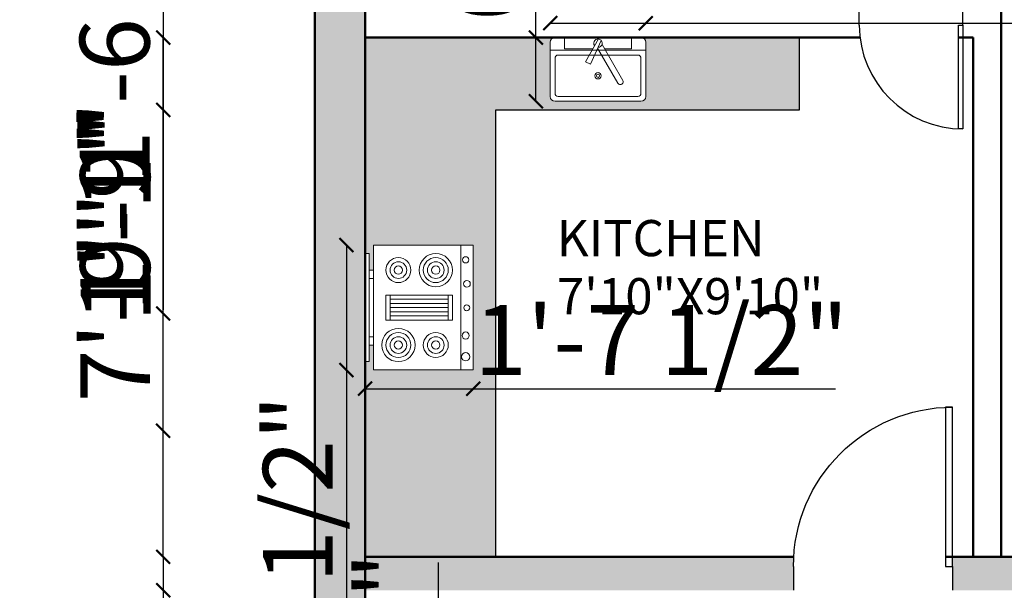
# Model space of a CAD drawing. Units: inches. Extents: x 2419 to 2878, y 1068 to 1713.
# Tile 14 of 20: x 2419 to 2595, y 1409 to 1511. Entities that reach past the tile are written whole.
import ezdxf

# ---------------------------------------------------------------- set-up
doc = ezdxf.new("R2010")
doc.units = ezdxf.units.IN
for name, color, linetype, lineweight in [('A-ANNO-DIMS', 2, 'Continuous', 18), ('A-AREA-IDEN', 7, 'Continuous', 18), ('A-DOOR', 4, 'Continuous', 25), ('A-EQPM', 9, 'Continuous', 18), ('A-FLOR-CASE', 8, 'Continuous', 25), ('A-FLOR-FIXT', 8, 'Continuous', 18), ('A-FLOR-PRKG-PATT', 1, 'Continuous', 13), ('A-FURN-PATT', 254, 'Continuous', 13), ('A-WALL', 7, 'Continuous', 50)]:
    doc.layers.add(name, color=color, linetype=linetype, lineweight=lineweight)
for name, color, linetype, lineweight, true_color in [('A-FLOR-CASE-PATT', 254, 'Continuous', 13, 0xcecce6), ('A-FLOR-FIXT-PATT', 254, 'Continuous', 13, 0xd7ebd2), ('A-WALL-PATT', 18, 'Continuous', 13, 0x000000)]:
    doc.layers.add(name, color=color, linetype=linetype, lineweight=lineweight, true_color=true_color)
doc.styles.get("Standard").update_dxf_attribs({"font": 'arial.ttf'})
doc.dimstyles.new('ISO-25', dxfattribs={"dimtxt": 12.5, "dimasz": 2.5, "dimexe": 1.25, "dimexo": 0.625, "dimtad": 1, "dimdec": 0, "dimlunit": 4, "dimtxsty": 'Standard', "dimblk": 'ARCHTICK', "dimcen": 2.5, "dimse1": 1, "dimse2": 1, "dimclrd": 4, "dimadec": 0, "dimazin": 0, "dimtfac": 1, "dimtdec": 0, "dimtmove": 0, "dimatfit": 3, "dimfxl": 1, "dimarcsym": 0})

# ---------------------------------------------------------------- blocks, each defined once
blk = doc.blocks.new('Range-Oven - 30 in top')
for p, q in [((0, -3), (30, -3)), ((12, -6), (18, -6)), ((13, -20), (13, -6)), ((14, -6), (14, -20)), ((15, -20), (15, -6)), ((16, -6), (16, -20)), ((17, -20), (17, -6)), ((18, -20), (12, -20)), ((6, -24), (6, -25)), ((8, -25), (8, -24)), ((22, -25), (22, -24)), ((24, -24), (24, -25))]:
    blk.add_line(p, q)
for points in [[(0, -24), (0, 0), (30, 0), (30, -24)], [(12, -21), (12, -5), (18, -5), (18, -21)], [(2, -26), (2, -25), (28, -25), (28, -26)]]:
    blk.add_lwpolyline(points, close=True)
for centre, radius in [((6, -9), 4), ((6, -9), 3), ((6, -9), 2), ((24, -9), 3), ((24, -9), 2), ((6, -9), 1), ((24, -9), 1), ((24, -18), 4), ((6, -18), 3), ((6, -18), 2), ((24, -18), 3), ((24, -18), 2), ((6, -18), 1), ((24, -18), 1)]:
    blk.add_circle(centre, radius)
blk = doc.blocks.new('Faucet - single handle top')
for p, q in [((0.08, -0.26), (-2.26, -4.34)), ((-1.37, -4.79), (0.55, -0.5)), ((4.43, -7.68), (0.72, -1.24)), ((-0.06, -1.9), (3.57, -8.18)), ((-2.26, -4.34), (-1.37, -4.79))]:
    blk.add_line(p, q)
for points in [[(-0.92, -2), (-6, -2), (-6, 0), (6, 0), (6, -2), (1.16, -2)], [(-0.01, -2), (-0.12, -2)]]:
    blk.add_lwpolyline(points)
for centre, radius, start, end in [((0, -1), 0.75, 269.2246, 216.2304), ((4, -7.93), 0.5, 210, 30)]:
    blk.add_arc(centre, radius, start, end)
blk = doc.blocks.new('Sink-single - 30 in top')
blk.add_line((-15, -3.999996), (15, -3.999996))
for points in [[(-13.5, 0), (13.5, 0)], [(-15, -18.499996), (-15, -1.5)], [(15, -1.5), (15, -18.499996)], [(-12.5, -5.499996), (12.5, -5.499996)], [(-13.5, -17.499996), (-13.5, -6.499996)], [(13.5, -6.499996), (13.5, -17.499996)], [(12.5, -18.499996), (-12.5, -18.499996)], [(13.5, -19.999996), (-13.5, -19.999996)]]:
    blk.add_lwpolyline(points)
for radius in [1, 0.5]:
    blk.add_circle((0, -11.999996), radius)
for centre, radius, start, end in [((-13.5, -1.5), 1.5, 90, 180), ((13.5, -1.5), 1.5, 0, 90), ((-12.5, -6.499996), 1, 90, 180), ((12.5, -6.499996), 1, 0, 90), ((-13.5, -18.499996), 1.5, 180, 270), ((-12.5, -17.499996), 1, 180, 270), ((12.5, -17.499996), 1, 270, 0), ((13.5, -18.499996), 1.5, 270, 0)]:
    blk.add_arc(centre, radius, start, end)
blk = doc.blocks.new('*U3')
for p, q in [((0, 0), (0, -6)), ((40, 0), (40, -6))]:
    blk.add_line(p, q)
blk.add_lwpolyline([(0, 0), (0, 40), (1.75, 40), (1.75, 0)], close=True)
blk.add_arc((0, 0), 40, 0, 90)
blk = doc.blocks.new('_ArchTick')
at = {"color": 0, "linetype": 'ByBlock', "const_width": 0.15}
blk.add_lwpolyline([(-0.5, -0.5), (0.5, 0.5)], dxfattribs=at)
blk = doc.blocks.new('*D22')
at = {"layer": 'A-ANNO-DIMS', "color": 4, "lineweight": -2, "transparency": 16777216}
for p, q in [((2513.7, 1510.38), (2530.82, 1510.38)), ((2530.82, 1510.38), (2656.31, 1510.38))]:
    blk.add_line(p, q, dxfattribs=at)
at = {"layer": 'Defpoints', "color": 0, "transparency": 16777216}
for p in [(2530.82, 1510.38), (2513.7, 1507.81), (2530.82, 1507.81)]:
    blk.add_point(p, dxfattribs=at)
at = {"layer": 'A-ANNO-DIMS', "color": 4, "lineweight": -2, "transparency": 16777216, "xscale": 2.5, "yscale": 2.5, "zscale": 2.5, "rotation": 180}
blk.add_blockref('_ArchTick', (2513.7, 1510.38), dxfattribs=at)
at = {"layer": 'A-ANNO-DIMS', "color": 4, "lineweight": -2, "transparency": 16777216, "xscale": 2.5, "yscale": 2.5, "zscale": 2.5}
blk.add_blockref('_ArchTick', (2530.82, 1510.38), dxfattribs=at)
at = {"layer": 'A-ANNO-DIMS', "color": 0, "transparency": 16777216, "insert": (2594.82, 1517.47), "char_height": 12.5, "attachment_point": 5}
blk.add_mtext('SINK 1\'-5" TYP.', dxfattribs=at)
blk = doc.blocks.new('*D23')
at = {"layer": 'A-ANNO-DIMS', "color": 4, "lineweight": -2, "transparency": 16777216}
for p, q in [((2511.14, 1507.81), (2511.14, 1626.6)), ((2511.14, 1496.4), (2511.14, 1507.81))]:
    blk.add_line(p, q, dxfattribs=at)
at = {"layer": 'Defpoints', "color": 0, "transparency": 16777216}
for p in [(2511.14, 1507.81), (2513.7, 1507.81), (2513.7, 1496.4)]:
    blk.add_point(p, dxfattribs=at)
at = {"layer": 'A-ANNO-DIMS', "color": 4, "lineweight": -2, "transparency": 16777216, "xscale": 2.5, "yscale": 2.5, "zscale": 2.5}
for p, rotation in [((2511.14, 1507.81), 90), ((2511.14, 1496.4), 270)]:
    blk.add_blockref('_ArchTick', p, dxfattribs=dict(at, rotation=rotation))
at = {"layer": 'A-ANNO-DIMS', "color": 0, "transparency": 16777216, "insert": (2504.05, 1568.45), "char_height": 12.5, "attachment_point": 5, "rotation": 90}
blk.add_mtext('0\'-11 1/2" TYP.', dxfattribs=at)
blk = doc.blocks.new('*D27')
at = {"layer": 'A-ANNO-DIMS', "color": 4, "lineweight": -2, "transparency": 16777216}
for p, q in [((2493.67, 1347.69), (2493.67, 1413.78)), ((2493.67, 1311.01), (2493.67, 1347.69))]:
    blk.add_line(p, q, dxfattribs=at)
at = {"layer": 'Defpoints', "color": 0, "transparency": 16777216}
for p in [(2493.67, 1347.69), (2502.77, 1347.69), (2502.77, 1311.01)]:
    blk.add_point(p, dxfattribs=at)
at = {"layer": 'A-ANNO-DIMS', "color": 4, "lineweight": -2, "transparency": 16777216, "xscale": 2.5, "yscale": 2.5, "zscale": 2.5}
for p, rotation in [((2493.67, 1347.69), 90), ((2493.67, 1311.01), 270)]:
    blk.add_blockref('_ArchTick', p, dxfattribs=dict(at, rotation=rotation))
at = {"layer": 'A-ANNO-DIMS', "color": 0, "transparency": 16777216, "insert": (2486.57, 1381.99), "char_height": 12.5, "attachment_point": 5, "rotation": 90}
blk.add_mtext('3\'-0 1/2"', dxfattribs=at)
blk = doc.blocks.new('*D28')
at = {"layer": 'A-ANNO-DIMS', "color": 4, "lineweight": -2, "transparency": 16777216}
for p, q in [((2477.16, 1470.63), (2477.16, 1448.27)), ((2477.16, 1448.27), (2477.16, 1306.15))]:
    blk.add_line(p, q, dxfattribs=at)
at = {"layer": 'Defpoints', "color": 0, "transparency": 16777216}
for p in [(2480.51, 1470.63), (2477.16, 1448.27), (2480.51, 1448.27)]:
    blk.add_point(p, dxfattribs=at)
at = {"layer": 'A-ANNO-DIMS', "color": 4, "lineweight": -2, "transparency": 16777216, "xscale": 2.5, "yscale": 2.5, "zscale": 2.5}
for p, rotation in [((2477.16, 1470.63), 90), ((2477.16, 1448.27), 270)]:
    blk.add_blockref('_ArchTick', p, dxfattribs=dict(at, rotation=rotation))
at = {"layer": 'A-ANNO-DIMS', "color": 0, "transparency": 16777216, "insert": (2470.07, 1375.96), "char_height": 12.5, "attachment_point": 5, "rotation": 90}
blk.add_mtext('RANGE 1\'-10 1/2"', dxfattribs=at)
blk = doc.blocks.new('*D29')
at = {"layer": 'A-ANNO-DIMS', "color": 4, "lineweight": -2, "transparency": 16777216}
for p, q in [((2480.51, 1444.92), (2499.89, 1444.92)), ((2499.89, 1444.92), (2564.82, 1444.92))]:
    blk.add_line(p, q, dxfattribs=at)
at = {"layer": 'Defpoints', "color": 0, "transparency": 16777216}
for p in [(2480.51, 1448.27), (2499.89, 1448.27), (2499.89, 1444.92)]:
    blk.add_point(p, dxfattribs=at)
at = {"layer": 'A-ANNO-DIMS', "color": 4, "lineweight": -2, "transparency": 16777216, "xscale": 2.5, "yscale": 2.5, "zscale": 2.5, "rotation": 180}
blk.add_blockref('_ArchTick', (2480.51, 1444.92), dxfattribs=at)
at = {"layer": 'A-ANNO-DIMS', "color": 4, "lineweight": -2, "transparency": 16777216, "xscale": 2.5, "yscale": 2.5, "zscale": 2.5}
blk.add_blockref('_ArchTick', (2499.89, 1444.92), dxfattribs=at)
at = {"layer": 'A-ANNO-DIMS', "color": 0, "transparency": 16777216, "insert": (2533.61, 1452.01), "char_height": 12.5, "attachment_point": 5}
blk.add_mtext('1\'-7 1/2"', dxfattribs=at)
blk = doc.blocks.new('*D48')
at = {"layer": 'A-ANNO-DIMS', "color": 4, "lineweight": -2, "transparency": 16777216}
for p, q in [((2444.31, 1567.55), (2444.31, 1548.96)), ((2444.31, 1548.96), (2444.31, 1484.03))]:
    blk.add_line(p, q, dxfattribs=at)
at = {"layer": 'Defpoints', "color": 0, "transparency": 16777216}
for p in [(2725.51, 1567.55), (2444.31, 1548.96), (2725.51, 1548.96)]:
    blk.add_point(p, dxfattribs=at)
at = {"layer": 'A-ANNO-DIMS', "color": 4, "lineweight": -2, "transparency": 16777216, "xscale": 2.5, "yscale": 2.5, "zscale": 2.5}
for p, rotation in [((2444.31, 1567.55), 90), ((2444.31, 1548.96), 270)]:
    blk.add_blockref('_ArchTick', p, dxfattribs=dict(at, rotation=rotation))
at = {"layer": 'A-ANNO-DIMS', "color": 0, "transparency": 16777216, "insert": (2437.23, 1515.25), "char_height": 12.5, "attachment_point": 5, "rotation": 90}
blk.add_mtext('1\'-6 1/2"', dxfattribs=at)
blk = doc.blocks.new('*D50')
at = {"layer": 'A-ANNO-DIMS', "color": 4, "lineweight": -2, "transparency": 16777216}
for p, q in [((2444.31, 1458.39), (2444.31, 1494.19)), ((2444.31, 1437.39), (2444.31, 1458.39))]:
    blk.add_line(p, q, dxfattribs=at)
at = {"layer": 'Defpoints', "color": 0, "transparency": 16777216}
for p in [(2444.31, 1458.39), (2763.51, 1458.39), (2763.51, 1437.39)]:
    blk.add_point(p, dxfattribs=at)
at = {"layer": 'A-ANNO-DIMS', "color": 4, "lineweight": -2, "transparency": 16777216, "xscale": 2.5, "yscale": 2.5, "zscale": 2.5}
for p, rotation in [((2444.31, 1458.39), 90), ((2444.31, 1437.39), 270)]:
    blk.add_blockref('_ArchTick', p, dxfattribs=dict(at, rotation=rotation))
at = {"layer": 'A-ANNO-DIMS', "color": 0, "transparency": 16777216, "insert": (2437.31, 1477.54), "char_height": 12.5, "attachment_point": 5, "rotation": 90}
blk.add_mtext('1\'-9"', dxfattribs=at)
blk = doc.blocks.new('*D55')
at = {"layer": 'A-ANNO-DIMS', "color": 4, "lineweight": -2, "transparency": 16777216}
for p, q in [((2444.31, 1414.81), (2444.31, 1408.81)), ((2444.31, 1408.81), (2444.31, 1371.83))]:
    blk.add_line(p, q, dxfattribs=at)
at = {"layer": 'Defpoints', "color": 0, "transparency": 16777216}
for p in [(2480.51, 1414.81), (2444.31, 1408.81), (2480.51, 1408.81)]:
    blk.add_point(p, dxfattribs=at)
at = {"layer": 'A-ANNO-DIMS', "color": 4, "lineweight": -2, "transparency": 16777216, "xscale": 2.5, "yscale": 2.5, "zscale": 2.5}
for p, rotation in [((2444.31, 1414.81), 90), ((2444.31, 1408.81), 270)]:
    blk.add_blockref('_ArchTick', p, dxfattribs=dict(at, rotation=rotation))
at = {"layer": 'A-ANNO-DIMS', "color": 0, "transparency": 16777216, "insert": (2437.31, 1389.07), "char_height": 12.5, "attachment_point": 5, "rotation": 90}
blk.add_mtext('0\'-6"', dxfattribs=at)
blk = doc.blocks.new('*D56')
at = {"layer": 'A-ANNO-DIMS', "color": 4, "lineweight": -2, "transparency": 16777216}
for p, q in [((2480.51, 1079.92), (2503.97, 1079.92)), ((2503.97, 1079.92), (2578.61, 1079.92))]:
    blk.add_line(p, q, dxfattribs=at)
at = {"layer": 'Defpoints', "color": 0, "transparency": 16777216}
for p in [(2480.51, 1507.81), (2503.97, 1494.85), (2503.97, 1079.92)]:
    blk.add_point(p, dxfattribs=at)
at = {"layer": 'A-ANNO-DIMS', "color": 4, "lineweight": -2, "transparency": 16777216, "xscale": 2.5, "yscale": 2.5, "zscale": 2.5, "rotation": 180}
blk.add_blockref('_ArchTick', (2480.51, 1079.92), dxfattribs=at)
at = {"layer": 'A-ANNO-DIMS', "color": 4, "lineweight": -2, "transparency": 16777216, "xscale": 2.5, "yscale": 2.5, "zscale": 2.5}
blk.add_blockref('_ArchTick', (2503.97, 1079.92), dxfattribs=at)
at = {"layer": 'A-ANNO-DIMS', "color": 0, "transparency": 16777216, "insert": (2542.54, 1087.01), "char_height": 12.5, "attachment_point": 5}
blk.add_mtext('1\'-11 1/2"', dxfattribs=at)
blk = doc.blocks.new('*D57')
at = {"layer": 'A-ANNO-DIMS', "color": 4, "lineweight": -2, "transparency": 16777216}
blk.add_line((2480.51, 1605.01), (2558.38, 1605.01), dxfattribs=at)
at = {"layer": 'Defpoints', "color": 0, "transparency": 16777216}
for p in [(2558.38, 1605.01), (2480.51, 1507.81), (2558.38, 1507.81)]:
    blk.add_point(p, dxfattribs=at)
at = {"layer": 'A-ANNO-DIMS', "color": 4, "lineweight": -2, "transparency": 16777216, "xscale": 2.5, "yscale": 2.5, "zscale": 2.5, "rotation": 180}
blk.add_blockref('_ArchTick', (2480.51, 1605.01), dxfattribs=at)
at = {"layer": 'A-ANNO-DIMS', "color": 4, "lineweight": -2, "transparency": 16777216, "xscale": 2.5, "yscale": 2.5, "zscale": 2.5}
blk.add_blockref('_ArchTick', (2558.38, 1605.01), dxfattribs=at)
at = {"layer": 'A-ANNO-DIMS', "color": 0, "transparency": 16777216, "insert": (2519.45, 1612.02), "char_height": 12.5, "attachment_point": 5}
blk.add_mtext('6\'-6"', dxfattribs=at)
blk = doc.blocks.new('*D58')
at = {"layer": 'A-ANNO-DIMS', "color": 4, "lineweight": -2, "transparency": 16777216}
for p, q in [((2444.31, 1507.81), (2444.31, 1494.85)), ((2444.31, 1494.85), (2444.31, 1459.05))]:
    blk.add_line(p, q, dxfattribs=at)
at = {"layer": 'Defpoints', "color": 0, "transparency": 16777216}
for p in [(2480.51, 1507.81), (2444.31, 1494.85), (2503.97, 1494.85)]:
    blk.add_point(p, dxfattribs=at)
at = {"layer": 'A-ANNO-DIMS', "color": 4, "lineweight": -2, "transparency": 16777216, "xscale": 2.5, "yscale": 2.5, "zscale": 2.5}
for p, rotation in [((2444.31, 1507.81), 90), ((2444.31, 1494.85), 270)]:
    blk.add_blockref('_ArchTick', p, dxfattribs=dict(at, rotation=rotation))
at = {"layer": 'A-ANNO-DIMS', "color": 0, "transparency": 16777216, "insert": (2437.41, 1475.7), "char_height": 12.5, "attachment_point": 5, "rotation": 90}
blk.add_mtext('1\'-1"', dxfattribs=at)
blk = doc.blocks.new('*D59')
at = {"layer": 'A-ANNO-DIMS', "color": 4, "lineweight": -2, "transparency": 16777216}
blk.add_line((2480.51, 1079.92), (2589.51, 1079.92), dxfattribs=at)
at = {"layer": 'Defpoints', "color": 0, "transparency": 16777216}
for p in [(2480.51, 1414.81), (2589.51, 1414.81), (2589.51, 1079.92)]:
    blk.add_point(p, dxfattribs=at)
at = {"layer": 'A-ANNO-DIMS', "color": 4, "lineweight": -2, "transparency": 16777216, "xscale": 2.5, "yscale": 2.5, "zscale": 2.5, "rotation": 180}
blk.add_blockref('_ArchTick', (2480.51, 1079.92), dxfattribs=at)
at = {"layer": 'A-ANNO-DIMS', "color": 4, "lineweight": -2, "transparency": 16777216, "xscale": 2.5, "yscale": 2.5, "zscale": 2.5}
blk.add_blockref('_ArchTick', (2589.51, 1079.92), dxfattribs=at)
at = {"layer": 'A-ANNO-DIMS', "color": 0, "transparency": 16777216, "insert": (2535.01, 1086.93), "char_height": 12.5, "attachment_point": 5}
blk.add_mtext('9\'-1"', dxfattribs=at)
blk = doc.blocks.new('*D60')
at = {"layer": 'A-ANNO-DIMS', "color": 4, "lineweight": -2, "transparency": 16777216}
blk.add_line((2444.31, 1414.81), (2444.31, 1507.81), dxfattribs=at)
at = {"layer": 'Defpoints', "color": 0, "transparency": 16777216}
for p in [(2444.31, 1507.81), (2480.51, 1507.81), (2480.51, 1414.81)]:
    blk.add_point(p, dxfattribs=at)
at = {"layer": 'A-ANNO-DIMS', "color": 4, "lineweight": -2, "transparency": 16777216, "xscale": 2.5, "yscale": 2.5, "zscale": 2.5}
for p, rotation in [((2444.31, 1507.81), 90), ((2444.31, 1414.81), 270)]:
    blk.add_blockref('_ArchTick', p, dxfattribs=dict(at, rotation=rotation))
at = {"layer": 'A-ANNO-DIMS', "color": 0, "transparency": 16777216, "insert": (2437.31, 1461.31), "char_height": 12.5, "attachment_point": 5, "rotation": 90}
blk.add_mtext('7\'-9"', dxfattribs=at)

msp = doc.modelspace()

# ---------------------------------------------------------------- hatches: boundary and pattern name
at = {"layer": 'A-FLOR-CASE-PATT'}
h = msp.add_hatch(color=256, dxfattribs=at)
h.dxf.hatch_style = 1
h.paths.add_polyline_path([(2503.97, 1494.85), (2558.38, 1494.85), (2558.38, 1507.81), (2529.96, 1507.81, -0.414214), (2530.82, 1506.96), (2530.82, 1497.26, -0.414214), (2529.96, 1496.4), (2514.56, 1496.4, -0.414214), (2513.7, 1497.26), (2513.7, 1506.96, -0.414214), (2514.56, 1507.81), (2480.51, 1507.81), (2480.51, 1469.14), (2481.26, 1469.14), (2481.26, 1466.16), (2482.01, 1466.16), (2482.01, 1470.63), (2499.89, 1470.63), (2499.89, 1448.27), (2482.01, 1448.27), (2482.01, 1452.74), (2481.26, 1452.74), (2481.26, 1449.76), (2480.51, 1449.76), (2480.51, 1414.81), (2503.97, 1414.81)])
at = {"layer": 'A-FLOR-FIXT-PATT'}
h = msp.add_hatch(color=256, dxfattribs=at)
h.dxf.hatch_style = 1
h.paths.add_polyline_path([(2771.51, 1458.39), (2763.51, 1458.39), (2763.51, 1437.39), (2771.51, 1437.39)])
h.paths.add_polyline_path([(2770.51, 1456.39, 0.5), (2769.51, 1457.39), (2765.51, 1457.39, 0.5), (2764.51, 1456.39), (2764.51, 1439.39, 0.5), (2765.51, 1438.39), (2769.51, 1438.39, 0.5), (2770.51, 1439.39)], flags=16)
h.paths.add_polyline_path([(2706.38, 1408.81), (2685.38, 1408.81), (2685.38, 1400.81), (2706.38, 1400.81)])
h.paths.add_polyline_path([(2704.38, 1401.81, 0.5), (2705.38, 1402.81), (2705.38, 1406.81, 0.5), (2704.38, 1407.81), (2687.38, 1407.81, 0.5), (2686.38, 1406.81), (2686.38, 1402.81, 0.5), (2687.38, 1401.81)], flags=16)
h.paths.add_polyline_path([(2574.48, 1207.45), (2633.94, 1207.45), (2633.94, 1217.37), (2574.48, 1217.37)], flags=9)
h.paths.add_polyline_path([(2574.45, 1217.83), (2610.47, 1217.83), (2610.47, 1227.88), (2574.45, 1227.88)], flags=9)
h.paths.add_polyline_path([(2672.43, 1304.02), (2718.62, 1304.02), (2718.62, 1313.94), (2672.43, 1313.94)], flags=9)
h.paths.add_polyline_path([(2672.4, 1314.4), (2750.13, 1314.4), (2750.13, 1324.45), (2672.4, 1324.45)], flags=9)
h.paths.add_polyline_path([(2500.43, 1374.44), (2544.8, 1374.44), (2544.8, 1384.36), (2500.43, 1384.36)], flags=9)
h.paths.add_polyline_path([(2500.41, 1384.82), (2566.08, 1384.82), (2566.08, 1394.87), (2500.41, 1394.87)], flags=9)
h.paths.add_polyline_path([(2738.93, 1376.75), (2778.27, 1376.75), (2778.27, 1386.67), (2738.93, 1386.67)], flags=9)
h.paths.add_polyline_path([(2659.12, 1357.8), (2703.49, 1357.8), (2703.49, 1367.72), (2659.12, 1367.72)], flags=9)
h.paths.add_polyline_path([(2659.1, 1368.18), (2694.11, 1368.18), (2694.11, 1378.23), (2659.1, 1378.23)], flags=9)
h.paths.add_polyline_path([(2730.12, 1466.07), (2769.46, 1466.07), (2769.46, 1475.99), (2730.12, 1475.99)], flags=9)
h.paths.add_polyline_path([(2730.1, 1476.45), (2765.12, 1476.45), (2765.12, 1486.5), (2730.1, 1486.5)], flags=9)
h.paths.add_polyline_path([(2730.38, 1518.65), (2761.48, 1518.65), (2761.48, 1528.57), (2730.38, 1528.57)], flags=9)
h.paths.add_polyline_path([(2730.36, 1529.03), (2780.96, 1529.03), (2780.96, 1539.07), (2730.36, 1539.07)], flags=9)
h.paths.add_polyline_path([(2629.32, 1455.19), (2688.78, 1455.19), (2688.78, 1465.11), (2629.32, 1465.11)], flags=9)
h.paths.add_polyline_path([(2629.3, 1465.57), (2681.9, 1465.57), (2681.9, 1475.62), (2629.3, 1475.62)], flags=9)
h.paths.add_polyline_path([(2513.23, 1456.48), (2562.63, 1456.48), (2562.63, 1466.4), (2513.23, 1466.4)], flags=9)
h.paths.add_polyline_path([(2513.21, 1466.86), (2556.26, 1466.86), (2556.26, 1476.91), (2513.21, 1476.91)], flags=9)
h.paths.add_polyline_path([(2488.87, 1521.54), (2519.97, 1521.54), (2519.97, 1531.46), (2488.87, 1531.46)], flags=9)
h.paths.add_polyline_path([(2536.55, 1543.51), (2580.92, 1543.51), (2580.92, 1553.43), (2536.55, 1553.43)], flags=9)
h.paths.add_polyline_path([(2536.56, 1553.92), (2573.53, 1553.92), (2573.53, 1563.8), (2536.56, 1563.8)], flags=9)
at = {"layer": 'A-FLOR-PRKG-PATT'}
h = msp.add_hatch(color=256, dxfattribs=at)
h.dxf.hatch_style = 1
edge = h.paths.add_edge_path()
edge.add_ellipse((2561.37, 1279.45), major_axis=(3.99, 0), ratio=0.842304, start_angle=0.6466, end_angle=90)
edge.add_line((2561.37, 1282.81), (2511.57, 1282.81))
edge.add_ellipse((2511.57, 1279.45), major_axis=(3.99, 0), ratio=0.842304, start_angle=90, end_angle=179.3534)
edge.add_ellipse((10560.89, 1188.62), major_axis=(-8054.03, 0), ratio=0.8423039, start_angle=-0.646554, end_angle=-0.628237)
edge.add_ellipse((2509.23, 1276.91), major_axis=(1.69, 0), ratio=0.842304, start_angle=179.3718, end_angle=248.4648)
edge.add_ellipse((10560.33, 1188.62), major_axis=(8052.29, 0), ratio=0.8423039, start_angle=179.353446, end_angle=179.381357, ccw=False)
edge.add_ellipse((2511.01, 1279.45), major_axis=(2.25, 0), ratio=0.842304, start_angle=90, end_angle=179.3534, ccw=False)
edge.add_line((2511.01, 1281.35), (2561.94, 1281.35))
edge.add_ellipse((2561.94, 1279.45), major_axis=(-2.25, 0), ratio=0.842304, start_angle=180.6466, end_angle=270, ccw=False)
edge.add_ellipse((-5487.38, 1188.62), major_axis=(8052.29, 0), ratio=0.8423039, start_angle=0.528271, end_angle=0.646554, ccw=False)
edge.add_ellipse((2563.71, 1276.91), major_axis=(-1.69, 0), ratio=0.842304, start_angle=111.5352, end_angle=180.6282)
edge.add_ellipse((-5487.95, 1188.62), major_axis=(-8054.03, 0), ratio=0.8423039, start_angle=180.628237, end_angle=180.646554)
edge = h.paths.add_edge_path()
edge.add_ellipse((2564.91, 1261.91), major_axis=(-1.12, 0), ratio=0.842304, start_angle=180, end_angle=270)
edge.add_line((2564.91, 1262.86), (2564.43, 1262.86))
edge.add_ellipse((-5487.38, 1188.62), major_axis=(8052.29, 0), ratio=0.8423039, start_angle=0.383867, end_angle=0.528271, ccw=False)
edge.add_line((2564.65, 1242.56), (2564.91, 1242.56))
edge.add_ellipse((2564.91, 1243.51), major_axis=(-1.12, 0), ratio=0.842304, start_angle=90, end_angle=180)
edge.add_line((2566.03, 1243.51), (2566.03, 1261.91))
edge = h.paths.add_edge_path()
edge.add_ellipse((2564.91, 1174.99), major_axis=(1.12, 0), ratio=0.842304, start_angle=0, end_angle=90)
edge.add_line((2564.91, 1175.94), (2564.89, 1175.94))
edge.add_ellipse((-5487.38, 1188.62), major_axis=(8052.29, 0), ratio=0.8423039, start_angle=-0.134987, end_angle=-0.090229, ccw=False)
edge.add_ellipse((2163.34, 1170.91), major_axis=(401.54, 0), ratio=0.842304, start_angle=-2.18, end_angle=-0.1356, ccw=False)
edge.add_line((2564.47, 1155.64), (2564.91, 1155.64))
edge.add_ellipse((2564.91, 1156.59), major_axis=(-1.12, 0), ratio=0.842304, start_angle=90, end_angle=180)
edge.add_line((2566.03, 1156.59), (2566.03, 1174.99))
h.paths.add_polyline_path([(2574.48, 1207.45), (2633.94, 1207.45), (2633.94, 1217.37), (2574.48, 1217.37)], flags=9)
h.paths.add_polyline_path([(2574.45, 1217.83), (2610.47, 1217.83), (2610.47, 1227.88), (2574.45, 1227.88)], flags=9)
h.paths.add_polyline_path([(2672.43, 1304.02), (2718.62, 1304.02), (2718.62, 1313.94), (2672.43, 1313.94)], flags=9)
h.paths.add_polyline_path([(2672.4, 1314.4), (2750.13, 1314.4), (2750.13, 1324.45), (2672.4, 1324.45)], flags=9)
h.paths.add_polyline_path([(2500.43, 1374.44), (2544.8, 1374.44), (2544.8, 1384.36), (2500.43, 1384.36)], flags=9)
h.paths.add_polyline_path([(2500.41, 1384.82), (2566.08, 1384.82), (2566.08, 1394.87), (2500.41, 1394.87)], flags=9)
h.paths.add_polyline_path([(2738.93, 1376.75), (2778.27, 1376.75), (2778.27, 1386.67), (2738.93, 1386.67)], flags=9)
h.paths.add_polyline_path([(2659.12, 1357.8), (2703.49, 1357.8), (2703.49, 1367.72), (2659.12, 1367.72)], flags=9)
h.paths.add_polyline_path([(2659.1, 1368.18), (2694.11, 1368.18), (2694.11, 1378.23), (2659.1, 1378.23)], flags=9)
h.paths.add_polyline_path([(2730.12, 1466.07), (2769.46, 1466.07), (2769.46, 1475.99), (2730.12, 1475.99)], flags=9)
h.paths.add_polyline_path([(2730.1, 1476.45), (2765.12, 1476.45), (2765.12, 1486.5), (2730.1, 1486.5)], flags=9)
h.paths.add_polyline_path([(2730.38, 1518.65), (2761.48, 1518.65), (2761.48, 1528.57), (2730.38, 1528.57)], flags=9)
h.paths.add_polyline_path([(2730.36, 1529.03), (2780.96, 1529.03), (2780.96, 1539.07), (2730.36, 1539.07)], flags=9)
h.paths.add_polyline_path([(2629.32, 1455.19), (2688.78, 1455.19), (2688.78, 1465.11), (2629.32, 1465.11)], flags=9)
h.paths.add_polyline_path([(2629.3, 1465.57), (2681.9, 1465.57), (2681.9, 1475.62), (2629.3, 1475.62)], flags=9)
h.paths.add_polyline_path([(2513.23, 1456.48), (2562.63, 1456.48), (2562.63, 1466.4), (2513.23, 1466.4)], flags=9)
h.paths.add_polyline_path([(2513.21, 1466.86), (2556.26, 1466.86), (2556.26, 1476.91), (2513.21, 1476.91)], flags=9)
h.paths.add_polyline_path([(2488.87, 1521.54), (2519.97, 1521.54), (2519.97, 1531.46), (2488.87, 1531.46)], flags=9)
h.paths.add_polyline_path([(2536.55, 1543.51), (2580.92, 1543.51), (2580.92, 1553.43), (2536.55, 1553.43)], flags=9)
h.paths.add_polyline_path([(2536.56, 1553.92), (2573.53, 1553.92), (2573.53, 1563.8), (2536.56, 1563.8)], flags=9)
at = {"layer": 'A-FURN-PATT'}
h = msp.add_hatch(color=256, dxfattribs=at)
h.dxf.hatch_style = 1
h.paths.add_polyline_path([(2710.17, 1562.64), (2707.17, 1559.64), (2709.17, 1559.64, -0.414214), (2710.17, 1560.64)])
h.paths.add_polyline_path([(2711.17, 1559.64, 1), (2709.17, 1559.64, 1)])
h.paths.add_polyline_path([(2710.17, 1562.64), (2710.17, 1560.64, -0.414214), (2711.17, 1559.64), (2713.17, 1559.64)])
h.paths.add_polyline_path([(2713.17, 1559.64), (2711.17, 1559.64, -0.414214), (2710.17, 1558.64), (2710.17, 1556.64)])
h.paths.add_polyline_path([(2710.17, 1558.64, -0.414214), (2709.17, 1559.64), (2707.17, 1559.64), (2710.17, 1556.64)])
h.paths.add_polyline_path([(2613.13, 1558.89, 1), (2611.13, 1558.89, 1)])
h.paths.add_polyline_path([(2612.13, 1561.89), (2612.13, 1559.89, -0.414214), (2613.13, 1558.89), (2615.13, 1558.89)])
h.paths.add_polyline_path([(2612.13, 1559.89), (2612.13, 1561.89), (2609.13, 1558.89), (2611.13, 1558.89, -0.414214)])
h.paths.add_polyline_path([(2612.13, 1557.89, -0.414214), (2611.13, 1558.89), (2609.13, 1558.89), (2612.13, 1555.89)])
h.paths.add_polyline_path([(2574.48, 1207.45), (2633.94, 1207.45), (2633.94, 1217.37), (2574.48, 1217.37)], flags=9)
h.paths.add_polyline_path([(2574.45, 1217.83), (2610.47, 1217.83), (2610.47, 1227.88), (2574.45, 1227.88)], flags=9)
h.paths.add_polyline_path([(2672.43, 1304.02), (2718.62, 1304.02), (2718.62, 1313.94), (2672.43, 1313.94)], flags=9)
h.paths.add_polyline_path([(2672.4, 1314.4), (2750.13, 1314.4), (2750.13, 1324.45), (2672.4, 1324.45)], flags=9)
h.paths.add_polyline_path([(2500.43, 1374.44), (2544.8, 1374.44), (2544.8, 1384.36), (2500.43, 1384.36)], flags=9)
h.paths.add_polyline_path([(2500.41, 1384.82), (2566.08, 1384.82), (2566.08, 1394.87), (2500.41, 1394.87)], flags=9)
h.paths.add_polyline_path([(2738.93, 1376.75), (2778.27, 1376.75), (2778.27, 1386.67), (2738.93, 1386.67)], flags=9)
h.paths.add_polyline_path([(2659.12, 1357.8), (2703.49, 1357.8), (2703.49, 1367.72), (2659.12, 1367.72)], flags=9)
h.paths.add_polyline_path([(2659.1, 1368.18), (2694.11, 1368.18), (2694.11, 1378.23), (2659.1, 1378.23)], flags=9)
h.paths.add_polyline_path([(2730.12, 1466.07), (2769.46, 1466.07), (2769.46, 1475.99), (2730.12, 1475.99)], flags=9)
h.paths.add_polyline_path([(2730.1, 1476.45), (2765.12, 1476.45), (2765.12, 1486.5), (2730.1, 1486.5)], flags=9)
h.paths.add_polyline_path([(2730.38, 1518.65), (2761.48, 1518.65), (2761.48, 1528.57), (2730.38, 1528.57)], flags=9)
h.paths.add_polyline_path([(2730.36, 1529.03), (2780.96, 1529.03), (2780.96, 1539.07), (2730.36, 1539.07)], flags=9)
h.paths.add_polyline_path([(2629.32, 1455.19), (2688.78, 1455.19), (2688.78, 1465.11), (2629.32, 1465.11)], flags=9)
h.paths.add_polyline_path([(2629.3, 1465.57), (2681.9, 1465.57), (2681.9, 1475.62), (2629.3, 1475.62)], flags=9)
h.paths.add_polyline_path([(2513.23, 1456.48), (2562.63, 1456.48), (2562.63, 1466.4), (2513.23, 1466.4)], flags=9)
h.paths.add_polyline_path([(2513.21, 1466.86), (2556.26, 1466.86), (2556.26, 1476.91), (2513.21, 1476.91)], flags=9)
h.paths.add_polyline_path([(2488.87, 1521.54), (2519.97, 1521.54), (2519.97, 1531.46), (2488.87, 1531.46)], flags=9)
h.paths.add_polyline_path([(2536.55, 1543.51), (2580.92, 1543.51), (2580.92, 1553.43), (2536.55, 1553.43)], flags=9)
h.paths.add_polyline_path([(2536.56, 1553.92), (2573.53, 1553.92), (2573.53, 1563.8), (2536.56, 1563.8)], flags=9)
at = {"layer": 'A-WALL-PATT'}
h = msp.add_hatch(color=256, dxfattribs=at)
h.dxf.hatch_style = 1
h.paths.add_polyline_path([(2780.51, 1577.81), (2471.51, 1577.81), (2471.51, 1121.81), (2780.51, 1121.81)])
h.paths.add_polyline_path([(2480.51, 1568.81), (2771.51, 1568.81), (2771.51, 1130.81), (2480.51, 1130.81)], flags=16)
h.paths.add_polyline_path([(2528.51, 1568.81), (2528.51, 1512.81), (2594.51, 1512.81), (2594.51, 1414.81), (2596.57, 1414.81), (2596.57, 1441.61), (2597.82, 1441.61), (2597.82, 1441.58, -0.384016), (2625.03, 1414.81), (2725.51, 1414.81), (2725.51, 1567.55), (2728.3, 1567.55), (2746.89, 1567.55), (2746.89, 1566.73), (2746.87, 1566.73, -0.367216), (2730.51, 1549.09), (2730.51, 1512.81), (2750.85, 1512.81), (2750.85, 1510.03, -0.401453), (2733.08, 1491.46), (2733.08, 1491.44), (2732.27, 1491.44), (2732.27, 1507.81), (2730.51, 1507.81), (2730.51, 1408.81), (2736.51, 1408.81), (2736.51, 1349.81), (2632.51, 1349.81), (2632.51, 1408.81), (2528.51, 1408.81), (2528.51, 1414.81), (2503.97, 1414.81), (2503.97, 1494.85), (2558.38, 1494.85), (2558.38, 1507.81), (2529.96, 1507.81, -0.414214), (2530.82, 1506.96), (2530.82, 1497.26, -0.414214), (2529.96, 1496.4), (2514.56, 1496.4, -0.414214), (2513.7, 1497.26), (2513.7, 1506.96, -0.414214), (2514.56, 1507.81), (2528.51, 1507.81), (2528.51, 1512.81), (2480.51, 1512.81)], flags=0)
h.paths.add_polyline_path([(2516.26, 1507.81), (2528.26, 1507.81), (2528.26, 1505.81), (2523.42, 1505.81), (2524.07, 1504.67), (2529.39, 1504.67, -0.414214), (2529.96, 1504.1), (2529.96, 1497.83, -0.414214), (2529.39, 1497.26), (2515.13, 1497.26, -0.414214), (2514.56, 1497.83), (2514.56, 1504.1, -0.414214), (2515.13, 1504.67), (2520.69, 1504.67), (2521.34, 1505.81), (2516.26, 1505.81)], flags=0)
h.paths.add_polyline_path([(2522.02, 1505.53), (2522.82, 1507.32, -0.65506), (2522.25, 1506.06), (2522.19, 1505.93), (2522.43, 1505.53)], flags=0)
h.paths.add_polyline_path([(2522.83, 1500.97, -1), (2521.69, 1500.97, -1)], flags=0)
h.paths.add_polyline_path([(2522.55, 1500.97, -1), (2521.98, 1500.97, -1)], flags=0)
h.paths.add_polyline_path([(2482.01, 1470.63), (2499.89, 1470.63), (2499.89, 1448.27), (2482.01, 1448.27), (2482.01, 1452.74), (2481.26, 1452.74), (2481.26, 1449.76), (2480.51, 1449.76), (2480.51, 1469.14), (2481.26, 1469.14), (2481.26, 1466.16), (2482.01, 1466.16)], flags=0)
h.paths.add_polyline_path([(2488.71, 1466.16, -1), (2484.24, 1466.16, -1)], flags=0)
h.paths.add_polyline_path([(2496.17, 1466.16, -1), (2490.2, 1466.16, -1)], flags=0)
h.paths.add_polyline_path([(2487.97, 1466.16, -1), (2484.99, 1466.16, -1)], flags=0)
h.paths.add_polyline_path([(2495.42, 1466.16, -1), (2490.95, 1466.16, -1)], flags=0)
h.paths.add_polyline_path([(2487.22, 1466.16, -1), (2485.73, 1466.16, -1)], flags=0)
h.paths.add_polyline_path([(2494.68, 1466.16, -1), (2491.69, 1466.16, -1)], flags=0)
h.paths.add_polyline_path([(2499.11, 1468, -1), (2497.98, 1468, -1)], flags=0)
h.paths.add_polyline_path([(2493.93, 1466.16, -1), (2492.44, 1466.16, -1)], flags=0)
h.paths.add_polyline_path([(2499.37, 1463.71, -1), (2498.17, 1463.71, -1)], flags=0)
h.paths.add_polyline_path([(2484.24, 1461.69), (2496.17, 1461.69), (2496.17, 1457.22), (2484.24, 1457.22)], flags=0)
h.paths.add_polyline_path([(2484.99, 1460.94), (2495.42, 1460.94), (2495.42, 1457.96), (2484.99, 1457.96)], flags=0)
h.paths.add_polyline_path([(2586.88, 1510.03), (2587.69, 1510.03), (2587.69, 1491.44), (2586.88, 1491.44)], flags=0)
h.paths.add_polyline_path([(2499.26, 1459.41, -1), (2498.2, 1459.41, -1)], flags=0)
h.paths.add_polyline_path([(2489.46, 1452.74, -1), (2483.5, 1452.74, -1)], flags=0)
h.paths.add_polyline_path([(2557.3, 1408.81), (2557.3, 1413.09, -0.401453), (2584.57, 1441.58), (2584.57, 1441.61), (2585.82, 1441.61), (2585.82, 1413.09), (2585.82, 1408.81)], flags=0)
h.paths.add_polyline_path([(2488.71, 1452.74, -1), (2484.24, 1452.74, -1)], flags=0)
h.paths.add_polyline_path([(2495.42, 1452.74, -1), (2490.95, 1452.74, -1)], flags=0)
h.paths.add_polyline_path([(2487.97, 1452.74, -1), (2484.99, 1452.74, -1)], flags=0)
h.paths.add_polyline_path([(2494.68, 1452.74, -1), (2491.69, 1452.74, -1)], flags=0)
h.paths.add_polyline_path([(2487.22, 1452.74, -1), (2485.73, 1452.74, -1)], flags=0)
h.paths.add_polyline_path([(2499.18, 1454.44, -1), (2497.9, 1454.44, -1)], flags=0)
h.paths.add_polyline_path([(2493.93, 1452.74, -1), (2492.44, 1452.74, -1)], flags=0)
h.paths.add_polyline_path([(2499.3, 1450.64, -1), (2497.79, 1450.64, -1)], flags=0)
h.paths.add_polyline_path([(2619.13, 1558.89, -1), (2605.13, 1558.89, -1)], flags=0)
h.paths.add_polyline_path([(2609.13, 1558.89), (2612.13, 1561.89), (2615.13, 1558.89), (2612.13, 1555.89)], flags=0)
h.paths.add_polyline_path([(2611.13, 1558.89, -1), (2613.13, 1558.89, -1)], flags=0)
h.paths.add_polyline_path([(2633.68, 1568.81), (2693.68, 1568.81), (2693.68, 1488.81), (2633.68, 1488.81)], flags=0)
h.paths.add_polyline_path([(2641.68, 1554.41), (2641.68, 1567.61), (2662.48, 1567.61), (2662.48, 1554.41), (2664.88, 1554.41), (2664.88, 1567.61), (2685.68, 1567.61), (2685.68, 1552.41), (2680.48, 1552.41), (2693.68, 1539.21), (2678.48, 1539.21), (2678.48, 1554.41)], flags=0)
h.paths.add_polyline_path([(2637.51, 1408.81), (2731.51, 1408.81), (2731.51, 1354.81), (2637.51, 1354.81), (2637.51, 1357.98), (2635.3, 1357.98), (2635.3, 1358.79), (2637.51, 1358.79)], flags=0)
h.paths.add_polyline_path([(2717.17, 1559.64, -1), (2703.17, 1559.64, -1)], flags=0)
h.paths.add_polyline_path([(2707.17, 1559.64), (2710.17, 1562.64), (2713.17, 1559.64), (2710.17, 1556.64)], flags=0)
h.paths.add_polyline_path([(2709.17, 1559.64, -1), (2711.17, 1559.64, -1)], flags=0)
h.paths.add_polyline_path([(2685.38, 1408.81), (2706.38, 1408.81), (2706.38, 1400.81), (2699.88, 1400.81), (2701.88, 1394.81, -0.501323), (2696.92, 1375.95, -0.132891), (2694.83, 1375.95, -0.501317), (2689.88, 1394.81), (2691.88, 1400.81), (2688.88, 1400.81), (2688.88, 1399.31), (2685.88, 1399.31), (2685.88, 1400.31), (2687.88, 1400.31), (2687.88, 1400.81), (2685.38, 1400.81)], flags=0)
h.paths.add_polyline_path([(2687.38, 1407.81), (2704.38, 1407.81, -0.5), (2705.38, 1406.81), (2705.38, 1402.81, -0.5), (2704.38, 1401.81), (2687.38, 1401.81, -0.5), (2686.38, 1402.81), (2686.38, 1406.81, -0.5)], flags=0)
h.paths.add_polyline_path([(2639.51, 1205.81), (2634.51, 1205.81), (2634.51, 1293.81), (2637.51, 1293.81), (2639.51, 1293.81)], flags=0)
h.paths.add_polyline_path([(2691.88, 1394.81), (2699.88, 1394.81, -0.48008), (2697.52, 1377.29, -0.215004), (2694.23, 1377.29, -0.48008)], flags=0)
h.paths.add_polyline_path([(2757.51, 1453.89), (2763.51, 1451.89), (2763.51, 1454.89), (2762.01, 1454.89), (2762.01, 1457.89), (2763.01, 1457.89), (2763.01, 1455.89), (2763.51, 1455.89), (2763.51, 1458.39), (2771.51, 1458.39), (2771.51, 1437.39), (2763.51, 1437.39), (2763.51, 1443.89), (2757.51, 1441.89, -0.501323), (2738.65, 1446.85, -0.132891), (2738.65, 1448.94, -0.501317)], flags=0)
h.paths.add_polyline_path([(2739.99, 1449.54, -0.48008), (2757.51, 1451.89), (2757.51, 1443.89, -0.48008), (2739.99, 1446.25, -0.215004)], flags=0)
h.paths.add_polyline_path([(2765.51, 1457.39), (2769.51, 1457.39, -0.5), (2770.51, 1456.39), (2770.51, 1439.39, -0.5), (2769.51, 1438.39), (2765.51, 1438.39, -0.5), (2764.51, 1439.39), (2764.51, 1456.39, -0.5)], flags=0)
h = msp.add_hatch(color=256, dxfattribs=at)
h.dxf.hatch_style = 1
h.paths.add_polyline_path([(2771.51, 1354.81), (2736.51, 1354.81), (2736.51, 1408.81), (2771.51, 1408.81), (2771.51, 1414.81), (2625.03, 1414.81, -0.015108), (2625.09, 1413.09), (2625.09, 1408.81), (2632.51, 1408.81), (2632.51, 1376.56), (2635.3, 1376.56, -0.029838), (2637.51, 1376.43), (2637.51, 1408.81), (2731.51, 1408.81), (2731.51, 1354.81), (2637.51, 1354.81), (2637.51, 1357.98), (2635.3, 1357.98), (2632.51, 1357.98), (2632.51, 1349.81), (2771.51, 1349.81)])
h.paths.add_polyline_path([(2639.51, 1298.81), (2637.51, 1298.81), (2480.51, 1298.81), (2480.51, 1293.81), (2637.51, 1293.81), (2639.51, 1293.81)])
h.paths.add_polyline_path([(2639.51, 1293.81), (2637.51, 1293.81), (2634.51, 1293.81), (2634.51, 1244.65), (2638.79, 1244.65, -0.006332), (2639.51, 1244.64)])
h.paths.add_polyline_path([(2639.51, 1205.81), (2771.51, 1205.81), (2771.51, 1210.81), (2639.51, 1210.81), (2639.51, 1216.13), (2638.79, 1216.13), (2634.51, 1216.13), (2634.51, 1130.81), (2639.51, 1130.81)])
h.paths.add_polyline_path([(2596.57, 1413.09), (2596.57, 1414.81), (2585.82, 1414.81), (2585.82, 1413.09), (2585.82, 1408.81), (2596.57, 1408.81)])
h.paths.add_polyline_path([(2557.3, 1413.09, -0.015108), (2557.35, 1414.81), (2480.51, 1414.81), (2480.51, 1408.81), (2557.3, 1408.81)])
h.paths.add_polyline_path([(2574.48, 1207.45), (2633.94, 1207.45), (2633.94, 1217.37), (2574.48, 1217.37)], flags=9)
h.paths.add_polyline_path([(2574.45, 1217.83), (2610.47, 1217.83), (2610.47, 1227.88), (2574.45, 1227.88)], flags=9)
h.paths.add_polyline_path([(2672.43, 1304.02), (2718.62, 1304.02), (2718.62, 1313.94), (2672.43, 1313.94)], flags=9)
h.paths.add_polyline_path([(2672.4, 1314.4), (2750.13, 1314.4), (2750.13, 1324.45), (2672.4, 1324.45)], flags=9)
h.paths.add_polyline_path([(2500.43, 1374.44), (2544.8, 1374.44), (2544.8, 1384.36), (2500.43, 1384.36)], flags=9)
h.paths.add_polyline_path([(2500.41, 1384.82), (2566.08, 1384.82), (2566.08, 1394.87), (2500.41, 1394.87)], flags=9)
h.paths.add_polyline_path([(2738.93, 1376.75), (2778.27, 1376.75), (2778.27, 1386.67), (2738.93, 1386.67)], flags=9)
h.paths.add_polyline_path([(2659.12, 1357.8), (2703.49, 1357.8), (2703.49, 1367.72), (2659.12, 1367.72)], flags=25)
h.paths.add_polyline_path([(2659.1, 1368.18), (2694.11, 1368.18), (2694.11, 1378.23), (2659.1, 1378.23)], flags=25)
h.paths.add_polyline_path([(2730.12, 1466.07), (2769.46, 1466.07), (2769.46, 1475.99), (2730.12, 1475.99)], flags=9)
h.paths.add_polyline_path([(2730.1, 1476.45), (2765.12, 1476.45), (2765.12, 1486.5), (2730.1, 1486.5)], flags=9)
h.paths.add_polyline_path([(2730.38, 1518.65), (2761.48, 1518.65), (2761.48, 1528.57), (2730.38, 1528.57)], flags=9)
h.paths.add_polyline_path([(2730.36, 1529.03), (2780.96, 1529.03), (2780.96, 1539.07), (2730.36, 1539.07)], flags=9)
h.paths.add_polyline_path([(2629.32, 1455.19), (2688.78, 1455.19), (2688.78, 1465.11), (2629.32, 1465.11)], flags=9)
h.paths.add_polyline_path([(2629.3, 1465.57), (2681.9, 1465.57), (2681.9, 1475.62), (2629.3, 1475.62)], flags=9)
h.paths.add_polyline_path([(2513.23, 1456.48), (2562.63, 1456.48), (2562.63, 1466.4), (2513.23, 1466.4)], flags=9)
h.paths.add_polyline_path([(2513.21, 1466.86), (2556.26, 1466.86), (2556.26, 1476.91), (2513.21, 1476.91)], flags=9)
h.paths.add_polyline_path([(2488.87, 1521.54), (2519.97, 1521.54), (2519.97, 1531.46), (2488.87, 1531.46)], flags=9)
h.paths.add_polyline_path([(2536.55, 1543.51), (2580.92, 1543.51), (2580.92, 1553.43), (2536.55, 1553.43)], flags=9)
h.paths.add_polyline_path([(2536.56, 1553.92), (2573.53, 1553.92), (2573.53, 1563.8), (2536.56, 1563.8)], flags=9)

# ---------------------------------------------------------------- linework, layer by layer
at = {"layer": 'A-EQPM'}
for centre, radius in [((2498.54, 1468), 0.565), ((2498.77, 1463.71), 0.603), ((2498.73, 1459.41), 0.528), ((2498.54, 1454.44), 0.64), ((2498.54, 1450.64), 0.754)]:
    msp.add_circle(centre, radius, dxfattribs=at)
at = {"layer": 'A-FLOR-CASE'}
for p, q in [((2558.38, 1494.85), (2558.38, 1507.81)), ((2503.97, 1414.81), (2503.97, 1494.85)), ((2503.97, 1494.85), (2558.38, 1494.85))]:
    msp.add_line(p, q, dxfattribs=at)
at = {"layer": 'A-WALL'}
for p, q in [((2480.51, 1130.81), (2480.51, 1568.81)), ((2594.51, 1414.81), (2594.51, 1568.81)), ((2480.51, 1507.81), (2569.24, 1507.81)), ((2586.88, 1507.81), (2589.51, 1507.81)), ((2589.51, 1414.81), (2589.51, 1507.81)), ((2480.51, 1414.81), (2557.35, 1414.81)), ((2584.57, 1414.81), (2597.82, 1414.81))]:
    msp.add_line(p, q, dxfattribs=at)
msp.add_lwpolyline([(2471.51, 1577.81), (2780.51, 1577.81), (2780.51, 1121.81), (2471.51, 1121.81)], close=True, dxfattribs=at)

# ---------------------------------------------------------------- block references
at = {"layer": 'A-DOOR', "xscale": 0.4646269055216028, "yscale": 0.4646269055216028, "zscale": 0.4646269055216028, "rotation": 180}
msp.add_blockref('*U3', (2587.69, 1510.03), dxfattribs=at)
at = {"layer": 'A-DOOR', "xscale": -0.712964811120882, "yscale": 0.712964811120882, "zscale": 0.712964811120882}
msp.add_blockref('*U3', (2585.82, 1413.09), dxfattribs=at)
at = {"layer": 'A-EQPM', "xscale": 0.7453559924999299, "yscale": 0.7453559924999299, "zscale": 0.7453559924999299, "rotation": 270}
msp.add_blockref('Range-Oven - 30 in top', (2499.89, 1470.63), dxfattribs=at)
at = {"layer": 'A-FLOR-FIXT', "xscale": 0.5705899714795267, "yscale": 0.5705899714795267, "zscale": 0.5705899714795267}
msp.add_blockref('Sink-single - 30 in top', (2522.26, 1507.81), dxfattribs=at)
at = {"layer": 'A-FLOR-FIXT'}
msp.add_blockref('Faucet - single handle top', (2522.26, 1507.81), dxfattribs=at)

# ---------------------------------------------------------------- texts
at = {"layer": 'A-AREA-IDEN'}
for s, height, p in [('KITCHEN', 6.475, (2514.88, 1468.65)), ('7\'10"X9\'10"', 6.4753, (2514.88, 1458.25))]:
    msp.add_text(s, height=height, dxfattribs=at).set_placement(p)

# ---------------------------------------------------------------- dimensions: what is measured, and where the dimension line sits
at = {"layer": 'A-ANNO-DIMS'}
for base, p1, p2, angle, text, picture, middle in [((2511.14, 1507.81), (2513.7, 1496.4), (2513.7, 1507.81), 90, '<> TYP.', '*D23', (2504.05, 1568.45)), ((2477.16, 1448.27), (2480.51, 1470.63), (2480.51, 1448.27), 270, 'RANGE <>', '*D28', (2470.07, 1375.96))]:
    dim = msp.add_linear_dim(base=base, p1=p1, p2=p2, angle=angle, text=text, dimstyle='ISO-25', override={"dimdec": 1, "dimlfac": 1, "dimrnd": 0, "dimzin": 1, "dimdsep": 46, "dimlunit": 4, "dimfrac": 2}, dxfattribs=at)
    dim.commit()
    dim.dimension.update_dxf_attribs({"geometry": picture, "text_midpoint": middle})
for base, p1, p2, picture, middle in [((2558.38, 1605.01), (2480.51, 1507.81), (2558.38, 1507.81), '*D57', (2519.45, 1612.02)), ((2503.97, 1079.92), (2480.51, 1507.81), (2503.97, 1494.85), '*D56', (2542.54, 1087.01)), ((2499.89, 1444.92), (2480.51, 1448.27), (2499.89, 1448.27), '*D29', (2533.61, 1452.01)), ((2589.51, 1079.92), (2480.51, 1414.81), (2589.51, 1414.81), '*D59', (2535.01, 1086.93))]:
    dim = msp.add_linear_dim(base=base, p1=p1, p2=p2, dimstyle='ISO-25', override={"dimdec": 1, "dimlfac": 1, "dimrnd": 0, "dimzin": 1, "dimdsep": 46, "dimlunit": 4, "dimfrac": 2}, dxfattribs=at)
    dim.commit()
    dim.dimension.update_dxf_attribs({"geometry": picture, "text_midpoint": middle})
for base, p1, p2, picture, middle in [((2444.31, 1548.96), (2725.51, 1567.55), (2725.51, 1548.96), '*D48', (2437.23, 1515.25)), ((2444.31, 1507.81), (2480.51, 1414.81), (2480.51, 1507.81), '*D60', (2437.31, 1461.31)), ((2444.31, 1494.85), (2480.51, 1507.81), (2503.97, 1494.85), '*D58', (2437.41, 1475.7)), ((2444.31, 1458.39), (2763.51, 1437.39), (2763.51, 1458.39), '*D50', (2437.31, 1477.54)), ((2444.31, 1408.81), (2480.51, 1414.81), (2480.51, 1408.81), '*D55', (2437.31, 1389.07)), ((2493.67, 1347.69), (2502.77, 1311.01), (2502.77, 1347.69), '*D27', (2486.57, 1381.99))]:
    dim = msp.add_linear_dim(base=base, p1=p1, p2=p2, angle=90, dimstyle='ISO-25', override={"dimdec": 1, "dimlfac": 1, "dimrnd": 0, "dimzin": 1, "dimdsep": 46, "dimlunit": 4, "dimfrac": 2}, dxfattribs=at)
    dim.commit()
    dim.dimension.update_dxf_attribs({"geometry": picture, "text_midpoint": middle})
dim = msp.add_linear_dim(base=(2530.82, 1510.38), p1=(2513.7, 1507.81), p2=(2530.82, 1507.81), text='SINK <> TYP.', dimstyle='ISO-25', override={"dimdec": 1, "dimlfac": 1, "dimrnd": 0, "dimzin": 1, "dimdsep": 46, "dimlunit": 4, "dimfrac": 2}, dxfattribs=at)
dim.commit()
dim.dimension.update_dxf_attribs({"geometry": '*D22', "text_midpoint": (2594.82, 1517.47)})

doc.saveas('drawing.dxf')
